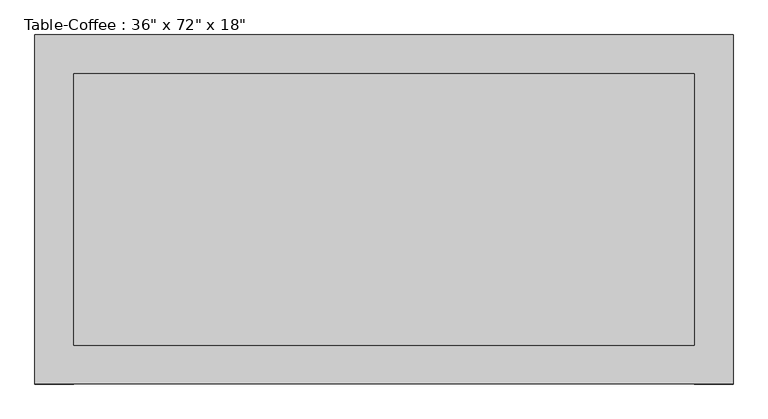
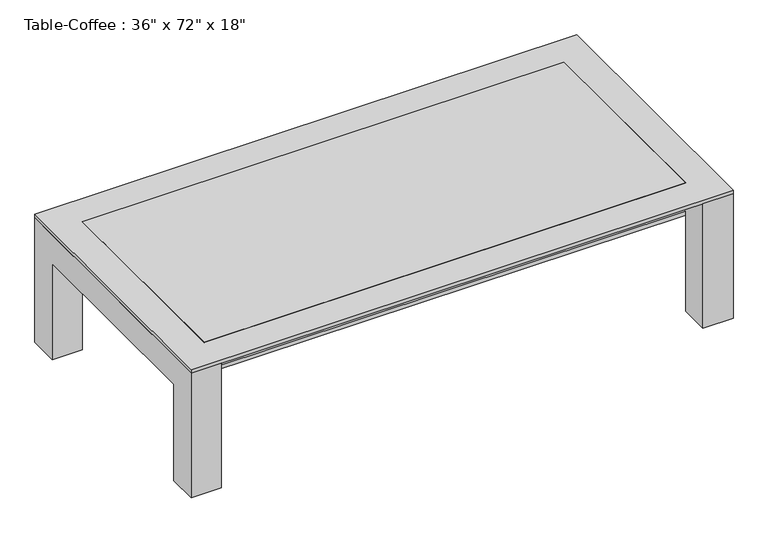
"""IFC4 building model written with IfcOpenShell, lengths in millimetres: furniture geometry."""

from ifc_helpers import new_model, si_unit, frame, origin, place, context, project, spatial, polyline, outline, extrude, source, transform, mapped, element, save


def furniture_cd93a443(model_context):
    return source(origin(), model_context, "Body", "SweptSolid", [
        extrude(outline(polyline([(831.0657667, 450.8110778), (831.0657667, -260.3889222), (-794.5342333, -260.3889222), (-794.5342333, 450.8110778), (831.0657667, 450.8110778)])), frame((0.0, 0.0, 342.9), z_axis=(0.0, 0.0, 1.0), x_axis=(1.0, 0.0, 0.0)), (0.0, 0.0, 1.0), 12.7),
        extrude(outline(polyline([(552.4110778, 0.0), (450.8110778, 0.0), (450.8110778, 342.9), (-260.3889222, 342.9), (-260.3889222, 0.0), (-361.9889222, 0.0), (-361.9889222, 444.5), (552.4110778, 444.5), (552.4110778, 0.0)])), frame((831.0657667, 0.0, 0.0), z_axis=(1.0, 0.0, 0.0), x_axis=(0.0, 1.0, 0.0)), (0.0, 0.0, 1.0), 101.6),
        extrude(outline(polyline([(552.4110778, 444.5), (552.4110778, 0.0), (450.8110778, 0.0), (450.8110778, 342.9), (-260.3889222, 342.9), (-260.3889222, 0.0), (-361.9889222, 0.0), (-361.9889222, 444.5), (552.4110778, 444.5)])), frame((-896.1342333, 0.0, 0.0), z_axis=(1.0, 0.0, 0.0), x_axis=(0.0, 1.0, 0.0)), (0.0, 0.0, 1.0), 101.6),
        extrude(outline(polyline([(831.0657667, 450.8110778), (831.0657667, -260.3889222), (-794.5342333, -260.3889222), (-794.5342333, 450.8110778), (831.0657667, 450.8110778)])), frame((0.0, 0.0, 444.5), z_axis=(0.0, 0.0, 1.0), x_axis=(1.0, 0.0, 0.0)), (0.0, 0.0, 1.0), 12.7),
        extrude(outline(polyline([(932.6657667, 552.4110778), (932.6657667, -361.9889222), (-896.1342333, -361.9889222), (-896.1342333, 552.4110778), (932.6657667, 552.4110778)]), holes=[polyline([(831.0657667, 450.8110778), (-794.5342333, 450.8110778), (-794.5342333, -260.3889222), (831.0657667, -260.3889222), (831.0657667, 450.8110778)])]), frame((0.0, 0.0, 444.5), z_axis=(0.0, 0.0, 1.0), x_axis=(1.0, 0.0, 0.0)), (0.0, 0.0, 1.0), 12.7),
    ])


if __name__ == "__main__":
    model = new_model("IFC4")
    model_context = context("Model", 3, world=origin())
    ifc_project = project(units=[si_unit("LENGTHUNIT", "METRE", prefix="MILLI")], contexts=[model_context])
    site = spatial("IfcSite", under=ifc_project)
    building = spatial("IfcBuilding", under=site)
    placement = place(None, origin())
    furniture_shape = furniture_cd93a443(model_context)
    element("IfcFurniture", 1, ObjectType="Table-Coffee : 36\" x 72\" x 18\"", at=placement, inside=building, context=model_context, shape_type="MappedRepresentation", body=[
        mapped(furniture_shape, transform((0.0, 0.0, 0.0), x_axis=(1.0, 0.0, 0.0), y_axis=(0.0, 1.0, 0.0), z_axis=(0.0, 0.0, 1.0))),
    ])
    save(model, "model.ifc")

# Revit data of these elements
# Type "Table-Coffee : 36\" x 72\" x 18\""
#   Assembly Code = "E2020200"
#   Height = 1' - 6"
#   Length = 6' - 0"
#   Width = 3' - 0"
#   Top Material = Steel, Chrome Plated
#   Frame Material = Wood - Teak
#   Default Elevation = 0
# Element 1 (IfcFurniture, "Table-Coffee : 36\" x 72\" x 18\"")
#   Materials on its faces: "Wood - Teak", "Steel, Chrome Plated", "Glass - Clear, Grey"
# Materials
#   "Steel, Chrome Plated": class "Metal", colour RGB 17 17 17, transparency 0, Description = "Chromiuim plated steel", Cost = 0
#   "Wood - Teak": class "Wood", colour RGB 120 73 19, transparency 0
#   "Glass - Clear, Grey": class "Glass", colour RGB 252 255 255, transparency 0.64
